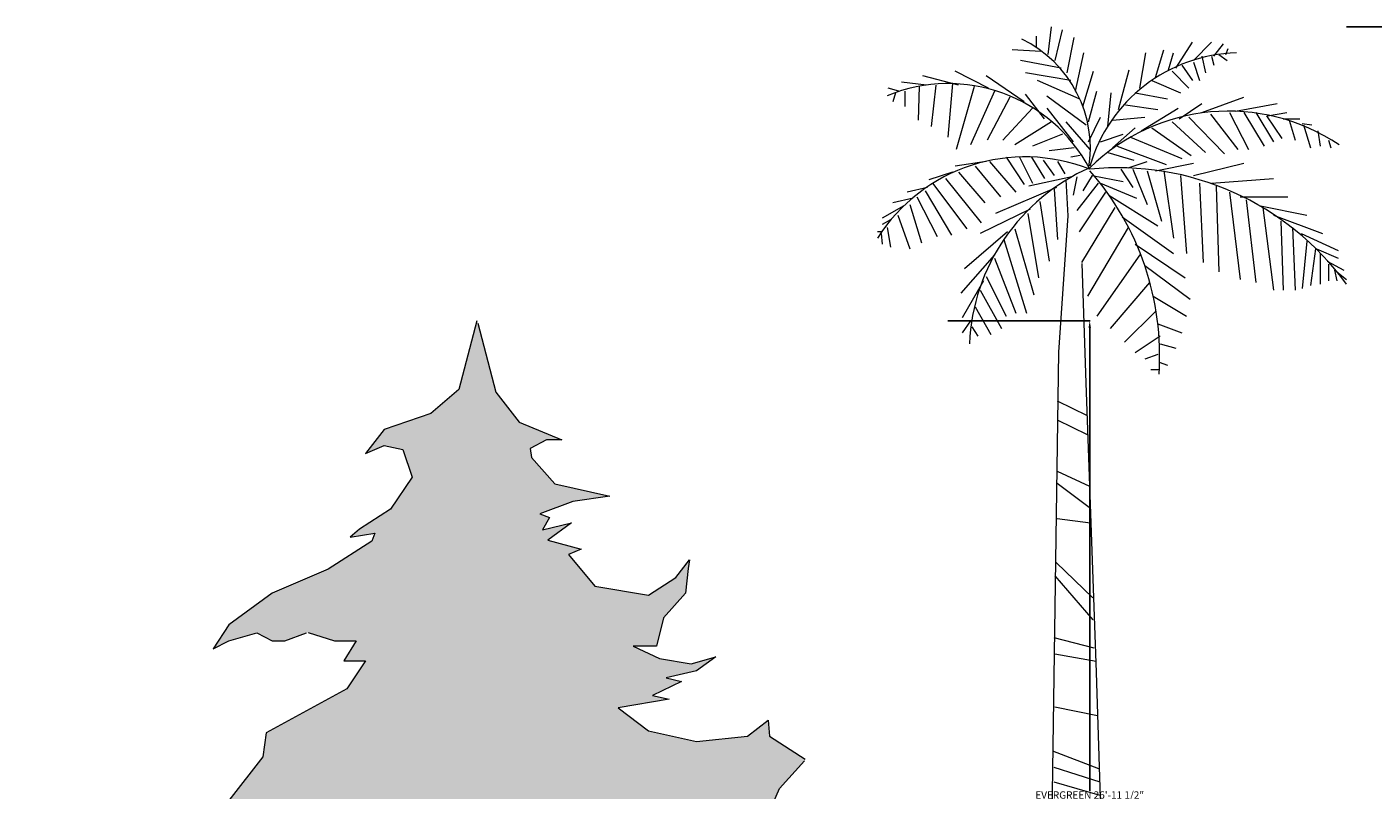
# Model space of a CAD drawing. Units: inches. Extents: x 481 to 2783, y 1975 to 3327.
# Tile 11 of 13: x 1872 to 2331, y 2286 to 2547. Entities that reach past the tile are written whole.
import ezdxf

# ---------------------------------------------------------------- set-up
doc = ezdxf.new("R2010")
doc.units = ezdxf.units.IN
doc.header["$MEASUREMENT"] = 0
doc.layers.add('A-ANNO-DIMS', color=50, linetype='Continuous', lineweight=18)
doc.layers.add('L-PLNT', color=7, linetype='Continuous', lineweight=13)
doc.layers.add('L-PLNT-PATT', color=116, linetype='Continuous', lineweight=13, true_color=0x136734)
doc.styles.get("Standard").update_dxf_attribs({"font": 'arial.ttf'})
doc.dimstyles.get("Standard").update_dxf_attribs({"dimtxt": 2.5, "dimasz": 2.5, "dimexe": 0.18, "dimexo": 0.0625, "dimgap": 0.09, "dimtad": 0, "dimtih": 1, "dimtoh": 1, "dimzin": 0, "dimdsep": 46, "dimlunit": 3, "dimtxsty": 'Standard', "dimcen": 0.09, "dimadec": 0, "dimazin": 0, "dimtfac": 1, "dimtofl": 0, "dimtmove": 0, "dimatfit": 3, "dimfxl": 1, "dimtolj": 1, "dimtzin": 0, "dimarcsym": 0})

# ---------------------------------------------------------------- blocks, each defined once
blk = doc.blocks.new('Tree - evergreen elevation')
for p, q in [((-8.263, 7.598), (-8.747, 14.105)), ((-0.771, 9.56), (-0.69, 11.833)), ((0, 0), (-0.771, 9.56)), ((-9.75, 0), (-8.263, 7.598))]:
    blk.add_line(p, q)
for points in [[(-3.9, 142.35), (-6.596, 132.037), (-10.801, 128.443), (-17.81, 126.047), (-20.614, 122.452), (-17.81, 123.65), (-15.007, 123.051), (-13.605, 118.858), (-16.876, 114.065), (-21.549, 111.07), (-22.951, 109.872), (-19.212, 110.471), (-19.68, 109.273), (-26.222, 105.079), (-34.633, 101.485), (-41.175, 96.693), (-43.511, 93.098), (-41.175, 94.296), (-36.969, 95.494), (-34.633, 94.296), (-32.764, 94.296), (-29.493, 95.494)], [(-3.759, 141.97), (-1.074, 131.643), (2.437, 127.141), (8.84, 124.493), (6.568, 124.493), (4.09, 123.169), (4.296, 121.846), (7.807, 117.874), (16.069, 116.02), (10.492, 115.226), (5.535, 113.372), (6.981, 112.843), (5.948, 110.989), (10.286, 112.048), (6.775, 109.401), (11.732, 108.077), (9.873, 107.282), (13.797, 102.516), (21.852, 101.192), (25.983, 103.84), (28.048, 106.488), (27.842, 105.164), (27.429, 101.457), (24.124, 97.75), (23.091, 93.513), (19.58, 93.513), (23.505, 91.66), (28.255, 90.866), (31.973, 91.925), (29.081, 89.806), (24.537, 88.747), (26.809, 88.218), (22.472, 86.099), (24.95, 85.57), (17.308, 84.246), (21.852, 80.804), (29.081, 79.215), (36.723, 80.009), (39.821, 82.392), (40.028, 80.009), (45.398, 76.567)], [(-29.25, 95.55), (-25.287, 94.296), (-22.016, 94.296), (-23.885, 91.301), (-20.614, 91.301), (-23.418, 87.108), (-35.567, 80.518), (-36.035, 76.924), (-41.175, 70.334), (-52.389, 65.542), (-58.931, 63.744), (-60.8, 61.348), (-57.062, 59.551), (-56.128, 60.749), (-50.987, 61.348), (-48.184, 57.754), (-40.707, 58.952), (-38.371, 62.546), (-30.427, 58.353), (-33.698, 58.353), (-35.1, 56.556), (-29.493, 54.159), (-30.894, 48.169), (-36.035, 41.579), (-44.446, 40.381), (-48.184, 33.791), (-49.118, 36.188), (-52.857, 32.593), (-59.399, 31.395), (-65.473, 31.395), (-70.146, 34.39), (-69.679, 30.796), (-66.875, 28.999), (-65.941, 27.202), (-61.268, 27.801), (-64.539, 22.409), (-58.464, 23.607), (-58.464, 18.815), (-54.258, 21.211), (-49.586, 21.81), (-50.987, 18.815), (-50.52, 15.82), (-47.249, 15.82), (-39.306, 18.216), (-36.502, 21.211), (-35.567, 15.82), (-30.427, 13.423), (-29.493, 15.221), (-25.287, 17.018), (-22.951, 15.221), (-21.081, 11.626), (-14.539, 15.82), (-13.138, 11.626), (-6.128, 15.82), (-4.726, 12.824), (10.226, 9.23), (5.554, 12.225), (13.497, 10.428), (10.226, 12.824), (16.768, 13.423), (22.376, 11.626), (27.516, 12.225), (21.909, 15.221), (34.993, 15.221), (44.806, 12.824), (41.535, 16.419), (42.469, 19.414), (49.011, 14.023), (56.487, 13.423), (66.768, 17.018), (64.431, 18.815), (60.226, 18.216), (60.226, 20.612), (56.955, 20.612), (56.955, 24.206), (54.151, 24.206), (51.348, 28.4), (50.413, 26.004), (47.609, 26.603), (43.871, 30.197), (38.731, 30.197), (34.525, 30.197), (27.983, 33.791), (38.731, 40.98), (47.609, 40.98), (45.273, 45.773), (52.282, 48.169), (56.955, 47.57), (55.086, 52.362), (48.544, 51.164), (39.198, 52.362), (35.927, 56.556), (33.123, 55.357), (31.254, 59.551), (27.049, 58.353), (22.376, 62.546), (28.451, 65.542), (39.198, 66.74), (41.535, 72.131), (45.273, 76.325)]]:
    blk.add_lwpolyline(points)
blk = doc.blocks.new('Tree - palm elevation')
for p, q in [((-5.567, 196.707), (-4.987, 201.167)), ((-4.407, 195.716), (-3.247, 200.672)), ((-7.5, 199.68), (-7.5, 197.946)), ((-2.474, 193.733), (-1.315, 199.433)), ((15.116, 194.477), (17.822, 198.689)), ((18.015, 195.716), (20.914, 198.689)), ((-6.727, 197.202), (-11.366, 197.45)), ((-1.121, 190.759), (0.232, 196.955)), ((9.317, 191.255), (10.283, 196.955)), ((11.829, 192.99), (13.182, 197.45)), ((13.956, 194.229), (14.729, 196.955)), ((19.368, 196.459), (19.948, 193.733)), ((20.914, 196.459), (21.301, 194.972)), ((21.301, 196.459), (22.847, 198.441)), ((22.074, 196.707), (23.427, 195.716)), ((23.234, 196.707), (23.62, 197.698)), ((-3.441, 194.477), (-10.013, 195.716)), ((5.837, 187.786), (7.577, 194.229)), ((16.082, 194.972), (17.822, 192.494)), ((18.015, 195.468), (18.981, 192.494)), ((-25.283, 191.751), (-29.342, 192.246)), ((-20.064, 191.751), (-25.863, 193.238)), ((-21.031, 191.998), (-21.804, 183.325)), ((-15.232, 191.255), (-20.644, 193.981)), ((-9.433, 189.025), (-15.618, 193.238)), ((-1.894, 192.494), (-9.24, 193.733)), ((-0.541, 189.52), (-7.307, 192.494)), ((0.038, 188.281), (1.778, 193.981)), ((11.25, 192.494), (15.889, 190.512)), ((14.536, 193.981), (17.242, 191.255)), ((-29.729, 190.759), (-31.469, 191.255)), ((-30.309, 190.512), (-30.695, 189.025)), ((-28.763, 190.759), (-28.763, 188.281)), ((-26.443, 191.503), (-26.636, 186.051)), ((-23.737, 191.751), (-24.51, 185.06)), ((-17.551, 191.503), (-20.451, 181.343)), ((-14.265, 190.759), (-18.131, 182.086)), ((-11.753, 189.768), (-15.425, 182.83)), ((-6.147, 186.299), (-9.24, 190.264)), ((-5.76, 190.016), (0.618, 185.308)), ((1.005, 185.803), (2.358, 190.759)), ((4.098, 185.06), (4.678, 190.512)), ((8.544, 190.512), (13.763, 189.52)), ((19.368, 187.29), (26.133, 189.768)), ((-8.08, 188.034), (-12.912, 182.83)), ((-5.76, 188.034), (-1.508, 182.582)), ((6.997, 188.529), (12.216, 187.786)), ((9.51, 184.317), (15.502, 188.034)), ((15.695, 186.299), (19.368, 188.777)), ((24.78, 187.538), (31.546, 188.777)), ((-4.987, 185.803), (-10.979, 182.086)), ((-2.668, 185.803), (1.198, 181.343)), ((1.005, 182.582), (2.938, 186.547)), ((4.871, 186.051), (10.09, 186.547)), ((14.536, 185.803), (19.948, 180.847)), ((17.242, 186.547), (23.041, 180.599)), ((20.721, 187.042), (25.167, 181.343)), ((23.814, 187.29), (26.907, 181.343)), ((26.133, 187.29), (29.419, 181.838)), ((28.066, 187.29), (30.966, 182.582)), ((29.806, 186.795), (32.319, 183.078)), ((29.999, 186.795), (33.092, 187.29)), ((32.512, 186.299), (35.218, 186.299)), ((33.479, 186.051), (34.445, 182.83)), ((35.605, 185.556), (37.151, 185.308)), ((-3.247, 183.821), (-8.08, 181.838)), ((2.938, 182.582), (6.61, 183.821)), ((4.871, 181.591), (8.544, 184.812)), ((7.77, 183.325), (16.082, 179.856)), ((11.25, 184.812), (17.628, 180.352)), ((35.798, 185.308), (36.958, 181.591)), ((38.118, 184.317), (38.504, 181.838)), ((-1.315, 181.591), (-5.374, 181.095)), ((5.644, 181.838), (13.569, 178.865)), ((39.857, 182.83), (40.244, 181.591)), ((-15.618, 179.36), (-20.644, 178.617)), ((-15.038, 179.36), (-10.786, 174.404)), ((-12.332, 180.104), (-9.433, 175.643)), ((-10.206, 180.104), (-8.08, 175.891)), ((-8.273, 180.104), (-6.147, 176.635)), ((-6.34, 179.608), (-4.6, 177.13)), ((-4.021, 179.36), (-2.861, 177.378)), ((-0.348, 180.352), (-1.894, 180.104)), ((4.098, 180.847), (8.35, 179.608)), ((7.384, 178.369), (10.476, 179.36)), ((11.829, 177.874), (18.015, 179.113)), ((18.015, 177.13), (26.133, 179.113)), ((-21.031, 177.626), (-24.897, 176.387)), ((-20.064, 177.626), (-15.812, 172.67)), ((-17.358, 178.617), (-13.299, 173.661)), ((-1.701, 176.882), (-8.66, 175.396)), ((-0.928, 176.882), (-1.508, 173.909)), ((1.585, 177.13), (0.038, 174.652)), ((1.585, 177.13), (6.61, 176.139)), ((6.224, 178.121), (8.157, 175.148)), ((8.157, 178.121), (10.476, 172.422)), ((10.476, 177.874), (12.796, 169.696)), ((13.182, 177.874), (14.729, 166.97)), ((15.889, 177.13), (16.855, 164.492)), ((-25.09, 175.148), (-28.376, 174.404)), ((-25.476, 174.652), (-21.224, 167.466)), ((-24.317, 175.891), (-18.711, 168.457)), ((-22.191, 176.635), (-16.391, 169.448)), ((-4.214, 175.148), (-14.072, 170.935)), ((-4.6, 174.9), (-4.021, 166.722)), ((-2.668, 176.387), (-2.376, 170.594)), ((2.551, 175.891), (-0.928, 171.431)), ((2.938, 175.891), (8.737, 173.413)), ((18.981, 175.891), (19.561, 163.005)), ((20.914, 175.891), (30.966, 176.635)), ((21.688, 175.396), (22.074, 161.518)), ((-27.409, 173.413), (-30.695, 172.67)), ((-27.989, 172.422), (-26.056, 166.227)), ((-26.829, 173.661), (-23.544, 167.218)), ((-6.92, 172.917), (-5.374, 163.253)), ((3.711, 174.404), (-0.541, 167.961)), ((4.291, 173.909), (12.216, 168.953)), ((23.814, 174.404), (25.554, 160.279)), ((25.554, 173.661), (33.285, 173.661)), ((26.52, 173.165), (28.066, 159.784)), ((-28.956, 172.174), (-32.435, 170.192)), ((-29.922, 170.687), (-27.989, 165.235)), ((-8.466, 171.678), (-16.585, 167.713)), ((-8.853, 170.935), (-7.113, 160.527)), ((5.257, 171.926), (-0.155, 163.005)), ((6.417, 170.439), (14.729, 164.492)), ((28.839, 172.174), (36.378, 170.687)), ((29.226, 171.926), (30.966, 158.545)), ((30.966, 170.687), (38.891, 167.713)), ((-32.628, 167.961), (-33.208, 167.961)), ((-31.082, 169.944), (-32.435, 169.2)), ((-31.662, 168.705), (-31.082, 165.483)), ((-12.139, 167.961), (-19.098, 162.014)), ((-10.979, 168.457), (-7.887, 157.801)), ((7.384, 168.705), (0.812, 157.553)), ((32.126, 169.696), (32.512, 158.545)), ((34.058, 168.705), (34.445, 158.545)), ((-32.628, 167.713), (-32.435, 165.979)), ((-12.719, 166.722), (-9.046, 154.828)), ((8.544, 165.979), (16.662, 160.527)), ((35.412, 167.713), (41.404, 164.988)), ((36.378, 166.474), (35.605, 158.792)), ((-14.265, 164.244), (-19.678, 158.049)), ((-14.265, 163.749), (-10.786, 154.828)), ((9.317, 164.244), (2.358, 154.332)), ((37.731, 165.235), (36.958, 159.288)), ((37.924, 165.235), (41.404, 163.749)), ((38.504, 164.492), (38.504, 159.536)), ((10.09, 162.51), (17.435, 157.058)), ((39.664, 163.253), (42.37, 161.766)), ((39.857, 162.757), (39.857, 160.031)), ((40.824, 161.766), (41.21, 160.031)), ((41.21, 161.518), (42.757, 160.279)), ((-16.005, 160.031), (-19.484, 154.084)), ((-15.618, 160.775), (-12.332, 154.332)), ((10.863, 159.784), (4.484, 152.35)), ((-16.585, 158.545), (-13.106, 152.35)), ((11.443, 157.553), (16.855, 154.332)), ((-17.358, 155.819), (-14.845, 151.358)), ((11.829, 155.075), (6.804, 150.119)), ((-18.131, 153.589), (-19.484, 151.606)), ((12.216, 153.093), (16.082, 151.606)), ((-17.938, 152.597), (-16.972, 151.111)), ((12.603, 151.111), (8.544, 148.385)), ((12.603, 149.872), (15.116, 149.128)), ((12.216, 148.137), (10.09, 147.393)), ((12.409, 146.898), (13.763, 146.402)), ((12.409, 145.659), (11.056, 145.659)), ((-4.081, 140.645), (0.753, 138.261)), ((-4.081, 137.547), (0.753, 135.163)), ((-4.081, 129.205), (1.124, 126.821)), ((-4.081, 127.298), (1.31, 123.246)), ((-4.081, 121.578), (1.31, 120.863)), ((-4.267, 114.428), (1.682, 108.708)), ((-4.453, 112.283), (1.682, 105.133)), ((-4.639, 102.273), (1.868, 100.604)), ((-4.453, 99.651), (2.24, 98.459)), ((-4.453, 91.071), (2.426, 89.641)), ((-4.825, 83.921), (2.612, 81.061)), ((-4.639, 81.299), (2.797, 78.916)), ((-4.639, 78.916), (2.797, 76.771))]:
    blk.add_line(p, q)
for points in [[(-2.363, 170.553), (-3.88, 148.505), (-4.988, 69.634), (-3.325, 24.869), (0, 0)], [(-0.116, 162.848), (0.554, 143.532), (2.217, 96.635), (3.88, 44.054), (7.76, 12.079), (11.64, 0)]]:
    blk.add_lwpolyline(points)
for centre, radius, start, end in [((-18.427, 181.448), 19.715, 350.285, 64.11229), ((25.595, 171.567), 25.395, 91.40319, 163.882), ((-21.738, 166.094), 25.899, 27.67115, 112.5305), ((23.687, 155.341), 32.188, 56.19272, 134.3213), ((-9.259, 151.732), 28.386, 68.38311, 147.5322), ((14.394, 148.393), 32.752, 113.7592, 177.4133), ((5.828, 132.718), 45.639, 35.98777, 95.82273), ((-32.8, 147.923), 45.309, 356.1943, 41.37848)]:
    blk.add_arc(centre, radius, start, end)
blk = doc.blocks.new('*D56')
at = {"layer": 'A-ANNO-DIMS', "color": 0, "lineweight": -2, "transparency": 16777216}
for p, q in [((2321.97, 2546.55), (2385.65, 2546.55)), ((2385.47, 2544.05), (2385.47, 2336.07)), ((2385.47, 2125.32), (2385.47, 2333.3)), ((2321.97, 2122.82), (2385.65, 2122.82))]:
    blk.add_line(p, q, dxfattribs=at)
at = {"layer": 'A-ANNO-DIMS', "color": 0, "transparency": 16777216}
for points in [[(2385.05, 2544.05), (2385.89, 2544.05), (2385.47, 2546.55)], [(2385.05, 2125.32), (2385.89, 2125.32), (2385.47, 2122.82)]]:
    blk.add_solid(points, dxfattribs=at)
at = {"layer": 'Defpoints', "color": 0, "transparency": 16777216}
for p in [(2321.91, 2546.55), (2385.47, 2546.55), (2321.91, 2122.82)]:
    blk.add_point(p, dxfattribs=at)
at = {"layer": 'A-ANNO-DIMS', "color": 0, "transparency": 16777216, "insert": (2385.47, 2334.69), "char_height": 2.5, "attachment_point": 5}
blk.add_mtext('\\A1;PALM 35\'-3 1/2"', dxfattribs=at)
blk = doc.blocks.new('*D62')
at = {"layer": 'A-ANNO-DIMS', "color": 0, "lineweight": -2, "transparency": 16777216}
for p, q in [((2185.87, 2446.33), (2234.51, 2446.33)), ((2234.33, 2443.83), (2234.33, 2285.96)), ((2234.33, 2125.32), (2234.33, 2283.19)), ((2185.87, 2122.82), (2234.51, 2122.82))]:
    blk.add_line(p, q, dxfattribs=at)
at = {"layer": 'A-ANNO-DIMS', "color": 0, "transparency": 16777216}
for points in [[(2233.91, 2443.83), (2234.75, 2443.83), (2234.33, 2446.33)], [(2233.91, 2125.32), (2234.75, 2125.32), (2234.33, 2122.82)]]:
    blk.add_solid(points, dxfattribs=at)
at = {"layer": 'Defpoints', "color": 0, "transparency": 16777216}
for p in [(2185.8, 2446.33), (2234.33, 2446.33), (2185.8, 2122.82)]:
    blk.add_point(p, dxfattribs=at)
at = {"layer": 'A-ANNO-DIMS', "color": 0, "transparency": 16777216, "insert": (2234.33, 2284.57), "char_height": 2.5, "attachment_point": 5}
blk.add_mtext('\\A1;EVERGREEN 26\'-11 1/2"', dxfattribs=at)

msp = doc.modelspace()

# ---------------------------------------------------------------- hatches: boundary and pattern name
at = {"layer": 'L-PLNT-PATT'}
h = msp.add_hatch(color=256, dxfattribs=at)
h.set_gradient(color1=(88, 186, 72), color2=(19, 155, 72))
h.paths.add_polyline_path([(2073.399, 2314.279), (2090.767, 2317.288), (2085.135, 2318.49), (2094.991, 2323.306), (2089.828, 2324.508), (2100.155, 2326.915), (2106.727, 2331.73), (2098.278, 2329.324), (2087.483, 2331.128), (2078.563, 2335.339), (2086.542, 2335.339), (2088.89, 2344.968), (2096.401, 2353.393), (2097.339, 2361.817), (2097.807, 2364.826), (2093.114, 2358.808), (2083.726, 2352.791), (2065.42, 2355.8), (2056.503, 2366.631), (2060.727, 2368.438), (2049.462, 2371.446), (2057.441, 2377.462), (2047.583, 2375.055), (2049.93, 2379.269), (2046.644, 2380.471), (2057.909, 2384.684), (2070.584, 2386.489), (2051.807, 2390.702), (2043.828, 2399.729), (2043.36, 2402.736), (2048.992, 2405.745), (2054.155, 2405.745), (2039.603, 2411.763), (2031.624, 2421.994), (2025.25, 2446.511), (2019.075, 2422.889), (2009.519, 2414.722), (1993.59, 2409.276), (1987.217, 2401.106), (1993.59, 2403.829), (1999.96, 2402.468), (2003.146, 2392.939), (1995.712, 2382.046), (1985.093, 2375.239), (1981.906, 2372.517), (1990.404, 2373.878), (1989.34, 2371.156), (1974.473, 2361.624), (1955.358, 2353.456), (1940.49, 2342.566), (1935.182, 2334.396), (1940.49, 2337.119), (1950.049, 2339.841), (1955.358, 2337.119), (1959.605, 2337.119), (1967.481, 2340.003), (1976.598, 2337.119), (1984.031, 2337.119), (1979.784, 2330.312), (1987.217, 2330.312), (1980.845, 2320.783), (1953.235, 2305.807), (1952.172, 2297.639), (1940.49, 2282.662), (1915.005, 2271.772), (1900.138, 2267.686), (1895.89, 2262.241), (1904.385, 2258.157), (1906.508, 2260.879), (1918.191, 2262.241), (1924.562, 2254.073), (1941.554, 2256.796), (1946.863, 2264.963), (1964.916, 2255.434), (1957.483, 2255.434), (1954.296, 2251.35), (1967.039, 2245.903), (1963.855, 2232.29), (1952.172, 2217.313), (1933.057, 2214.591), (1924.562, 2199.614), (1922.439, 2205.062), (1913.942, 2196.892), (1899.074, 2194.169), (1885.27, 2194.169), (1874.651, 2200.976), (1875.712, 2192.808), (1882.084, 2188.724), (1884.207, 2184.64), (1894.827, 2186.001), (1887.393, 2173.748), (1901.199, 2176.47), (1901.199, 2165.58), (1910.758, 2171.025), (1921.375, 2172.386), (1918.191, 2165.58), (1919.253, 2158.773), (1926.686, 2158.773), (1944.738, 2164.218), (1951.11, 2171.025), (1953.235, 2158.773), (1964.916, 2153.326), (1967.039, 2157.412), (1976.598, 2161.496), (1981.906, 2157.412), (1986.156, 2149.242), (2001.024, 2158.773), (2004.208, 2149.242), (2020.139, 2158.773), (2023.325, 2151.965), (2057.305, 2143.797), (2046.687, 2150.603), (2064.738, 2146.519), (2057.305, 2151.965), (2072.172, 2153.326), (2084.917, 2149.242), (2096.598, 2150.603), (2083.856, 2157.412), (2113.591, 2157.412), (2135.892, 2151.965), (2128.458, 2160.135), (2130.581, 2166.941), (2145.448, 2154.689), (2162.438, 2153.326), (2185.803, 2161.496), (2180.492, 2165.58), (2170.935, 2164.218), (2170.935, 2169.664), (2163.502, 2169.664), (2163.502, 2177.831), (2157.129, 2177.831), (2150.759, 2187.363), (2148.634, 2181.918), (2142.262, 2183.279), (2133.767, 2191.447), (2122.086, 2191.447), (2112.527, 2191.447), (2097.66, 2199.614), (2122.086, 2215.952), (2142.262, 2215.952), (2136.953, 2226.845), (2152.882, 2232.29), (2163.502, 2230.929), (2159.254, 2241.819), (2144.387, 2239.096), (2123.147, 2241.819), (2115.713, 2251.35), (2109.341, 2248.625), (2105.093, 2258.157), (2095.537, 2255.434), (2084.917, 2264.963), (2098.723, 2271.772), (2123.147, 2274.495), (2128.458, 2286.746), (2137.368, 2296.744), (2125.033, 2304.65), (2124.563, 2310.066), (2117.522, 2304.65), (2100.155, 2302.845), (2083.726, 2306.457)])
h.paths.add_polyline_path([(726.446, 2320.727), (718.597, 2319.609), (709.875, 2314.018), (699.409, 2308.428), (698.537, 2312.9), (690.688, 2296.128), (704.642, 2299.483), (713.364, 2293.892), (710.747, 2280.475), (695.049, 2274.884), (688.071, 2279.357), (685.455, 2272.648), (679.35, 2271.53), (674.117, 2264.821), (668.011, 2256.995), (675.861, 2250.286), (681.094, 2253.64), (675.177, 2243.917), (679.476, 2244.418), (678.855, 2235.617), (664.523, 2216.742), (647.08, 2215.624), (639.23, 2211.152), (626.148, 2196.616), (631.381, 2187.671), (663.651, 2188.789), (669.756, 2184.317), (684.583, 2191.026), (695.049, 2168.663), (699.409, 2168.663), (719.469, 2193.262), (725.574, 2196.616), (729.935, 2191.026), (729.935, 2183.199), (736.912, 2180.963), (746.506, 2180.963), (749.995, 2188.789), (761.333, 2194.38), (772.671, 2195.498), (777.904, 2199.971), (778.776, 2201.089), (781.392, 2206.679), (784.881, 2204.443), (787.498, 2195.498), (793.603, 2198.852), (795.347, 2196.616), (797.091, 2191.026), (803.197, 2201.089), (809.302, 2201.089), (811.918, 2196.616), (809.302, 2192.144), (816.279, 2194.38), (818.895, 2191.026), (825, 2195.498), (831.106, 2193.262), (843.316, 2180.963), (848.549, 2178.726), (852.91, 2174.254), (889.54, 2177.608), (896.518, 2170.9), (901.751, 2173.136), (887.796, 2191.026), (886.924, 2197.734), (891.285, 2204.443), (883.435, 2225.687), (879.075, 2225.687), (870.353, 2256.995), (861.631, 2258.112), (866.864, 2262.585), (873.841, 2280.475), (859.887, 2295.01), (842.444, 2300.601), (850.293, 2312.9), (843.316, 2334.144), (838.955, 2334.144), (830.233, 2353.152), (825, 2352.034), (818.895, 2352.034), (814.534, 2360.979), (817.151, 2373.278), (824.128, 2373.278), (811.046, 2388.932), (809.286, 2401.34), (802.324, 2409.058), (796.219, 2402.35), (792.731, 2404.586), (791.858, 2410.176), (787.498, 2412.413), (781.392, 2406.822), (774.415, 2407.94), (769.182, 2397.877), (769.182, 2388.932), (776.16, 2385.578), (770.926, 2382.223), (765.694, 2386.696), (750.867, 2372.16), (750.867, 2368.806), (744.762, 2365.452), (746.506, 2362.097), (750.867, 2355.389), (743.017, 2349.798), (735.168, 2355.389), (730.807, 2354.271), (729.063, 2349.798), (735.168, 2348.68), (736.04, 2339.735), (729.221, 2340.853), (721.213, 2333.026), (729.935, 2331.908)])

# ---------------------------------------------------------------- block references
at = {"layer": 'L-PLNT'}
for name, p, xscale, yscale, zscale in [('Tree - palm elevation', (2231.847, 2122.821), 2.106372464461094, 2.106372464461094, 2.106372464461094), ('Tree - evergreen elevation', (2034.065, 2122.821), 2.272610793994812, 2.272610793994812, 2.272610793994812)]:
    msp.add_blockref(name, p, dxfattribs=dict(at, xscale=xscale, yscale=yscale, zscale=zscale))

# ---------------------------------------------------------------- dimensions: what is measured, and where the dimension line sits
at = {"layer": 'A-ANNO-DIMS'}
for base, p1, p2, text, picture, middle in [((2385.469, 2546.553), (2321.909, 2122.821), (2321.909, 2546.553), 'PALM <>', '*D56', (2385.469, 2334.687)), ((2234.329, 2446.327), (2185.803, 2122.821), (2185.803, 2446.327), 'EVERGREEN <>', '*D62', (2234.329, 2284.574))]:
    dim = msp.add_linear_dim(base=base, p1=p1, p2=p2, angle=90, text=text, dimstyle='Standard', override={"dimdec": 1, "dimlfac": 1, "dimrnd": 0, "dimzin": 1, "dimdsep": 46, "dimlunit": 4, "dimfrac": 2}, dxfattribs=at)
    dim.commit()
    dim.dimension.update_dxf_attribs({"geometry": picture, "text_midpoint": middle})

doc.saveas('drawing.dxf')
